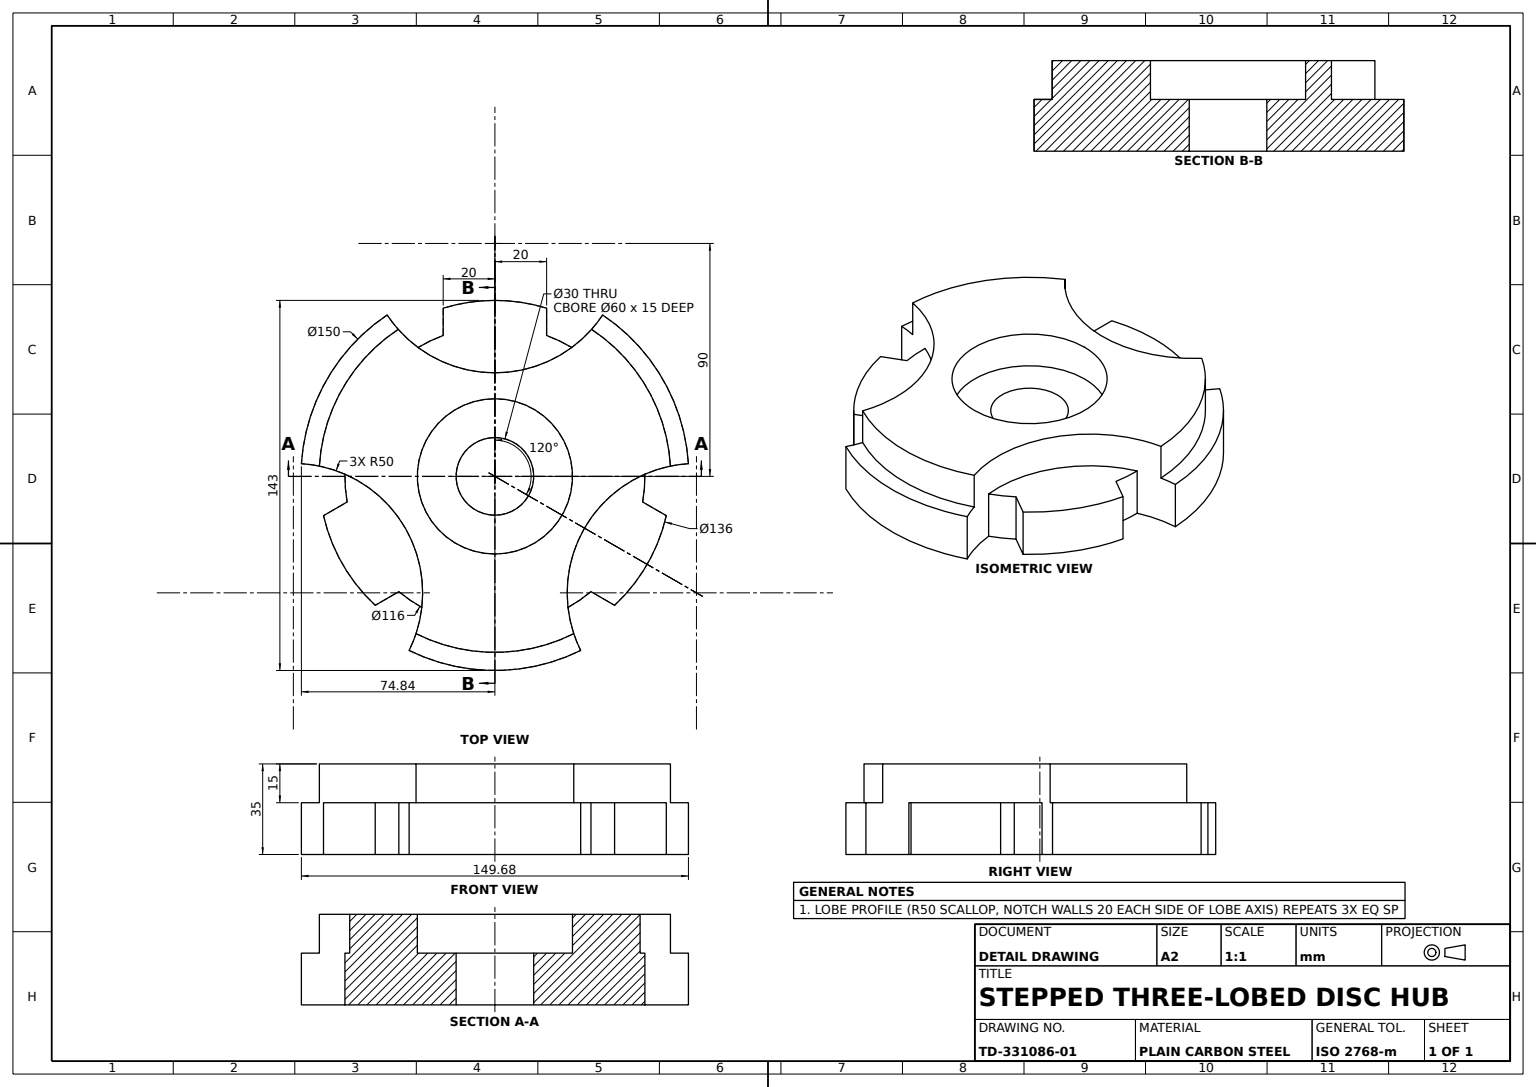
SolidWorks part; units mm, degrees
material "Plain Carbon Steel"
ref_plane "Front Plane" through (0, 0, 0) normal (0, 0, 1) x (1, 0, 0)
ref_plane "Top Plane" through (0, 0, 0) normal (0, 1, 0) x (1, 0, 0)
ref_plane "Right Plane" through (0, 0, 0) normal (1, 0, 0) x (0, 0, -1)
sketch "Base Lobe Profile Sketch" plane through (0, 0, 0) normal (0, 1, 0) x (1, 0, 0)
  line L0 (0, 40) -> (0, 81.413) construction
  line L1 (20, 54.4426) -> (20, 64.9923)
  line L2 (-20, 54.4426) -> (-20, 64.9923)
  line L3 (37.1487, -44.5418) -> (46.285, -49.8167)
  line L4 (-20, 40) -> (-20, 81.413) construction
  line L5 (20, 40) -> (20, 81.413) construction
  line L6 (57.1487, -9.9008) -> (66.285, -15.1756)
  line L7 (-57.1487, -9.9008) -> (-66.285, -15.1756)
  line L8 (-37.1487, -44.5418) -> (-46.285, -49.8167)
  arc A0 (-41.6664, 62.3611) -> (-74.8395, 4.9036) centre (0, 0) ccw
  circle A1 centre (0, 0) radius 90 construction
  arc A2 (-41.6664, 62.3611) -> (41.6664, 62.3611) centre (0, 90) ccw
  arc A3 (74.8395, 4.9036) -> (33.1731, -67.2647) centre (77.9423, -45) ccw
  arc A4 (-33.1731, -67.2647) -> (-74.8395, 4.9036) centre (-77.9423, -45) ccw
  arc A5 (-33.1731, -67.2647) -> (33.1731, -67.2647) centre (0, 0) ccw
  arc A6 (74.8395, 4.9036) -> (41.6664, 62.3611) centre (0, 0) ccw
  arc A7 (20, 64.9923) -> (-20, 64.9923) centre (0, 0) ccw
  arc A8 (-20, 54.4426) -> (-29.7315, 49.8) centre (0, 0) ccw
  arc A10 (-37.1487, -44.5418) -> (-28.2623, -50.6482) centre (0, 0) ccw
  arc A11 (57.1487, -9.9008) -> (57.9938, 0.8482) centre (0, 0) ccw
  arc A12 (-66.285, -15.1756) -> (-46.285, -49.8167) centre (0, 0) ccw
  arc A13 (46.285, -49.8167) -> (66.285, -15.1756) centre (0, 0) ccw
  arc A14 (28.2623, -50.6482) -> (37.1487, -44.5418) centre (0, 0) ccw
  arc A15 (29.7315, 49.8) -> (20, 54.4426) centre (0, 0) ccw
  arc A16 (-57.9938, 0.8482) -> (-57.1487, -9.9008) centre (0, 0) ccw
  dimension "D1" = 150
  dimension "D2" = 180
  dimension "D3" = 100
  dimension "D5" = 136
  dimension "D8" = 116
  dimension "D9" = 3
  dimension "D6" = 20
  dimension "D7" = 20
  dimension "D4" = 3
extrude "Base Lobe Plate 20mm" add sketch "Base Lobe Profile Sketch" along normal blind 20 contours A3 A6 A2 A0 A4 A5 | A4 A16 L7 A12 L8 A10 | A3 A14 L3 A13 L6 A11 | A2 A15 L1 A7 L2 A8
sketch "Upper Lobe Profile Sketch" plane through (0, 20, 0) normal (0, 1, 0) x (1, 0, 0)
  arc A0 (67.8836, 3.9778) -> (37.3866, 56.8) centre (0, 0) ccw
  circle A1 centre (0, 0) radius 90 construction
  arc A2 (-37.3866, 56.8) -> (37.3866, 56.8) centre (0, 90) ccw
  arc A3 (89.9303, 3.5416) -> (30.4969, -60.7778) centre (77.9423, -45) ccw
  arc A4 (-30.4969, -60.7778) -> (-67.8836, 3.9778) centre (-77.9423, -45) ccw
  arc A5 (-30.4969, -60.7778) -> (30.4969, -60.7778) centre (0, 0) ccw
  arc A6 (-37.3866, 56.8) -> (-67.8836, 3.9778) centre (0, 0) ccw
  arc M2 (57.9938, 0.8482) -> (74.8395, 4.9036) centre (77.9423, -45) cw
  arc M4 (41.6664, 62.3611) -> (29.7315, 49.8) centre (0, 90) cw
  arc M10 (-29.7315, 49.8) -> (-41.6664, 62.3611) centre (0, 90) cw
  arc M12 (-74.8395, 4.9036) -> (-57.9938, 0.8482) centre (-77.9423, -45) cw
  arc M18 (-28.2623, -50.6482) -> (-33.1731, -67.2647) centre (-77.9423, -45) cw
  arc M20 (33.1731, -67.2647) -> (28.2623, -50.6482) centre (77.9423, -45) cw
  dimension "D1" = 180
  dimension "D2" = 136
  dimension "D3" = 100
  dimension "D4" = 3
extrude "Upper Lobe Boss 15mm" add sketch "Upper Lobe Profile Sketch" along normal blind 15 contours A6 A4 A5 A3 A0 A2 M10 M12 M18 M20 M2 M4
sketch "Counterbore Sketch Ø60" plane through (0, 35, 0) normal (0, 1, 0) x (1, 0, 0)
  circle A0 centre (0, 0) radius 30
  dimension "D1" = 60
extrude "Counterbore Ø60x15" cut sketch "Counterbore Sketch Ø60" against normal blind 15
sketch "Through Hole Sketch Ø30" plane through (0, 20, 0) normal (0, 1, 0) x (1, 0, 0)
  circle A0 centre (0, 0) radius 15
  dimension "D1" = 30
extrude "Through Hole Ø30" cut sketch "Through Hole Sketch Ø30" against normal through all
